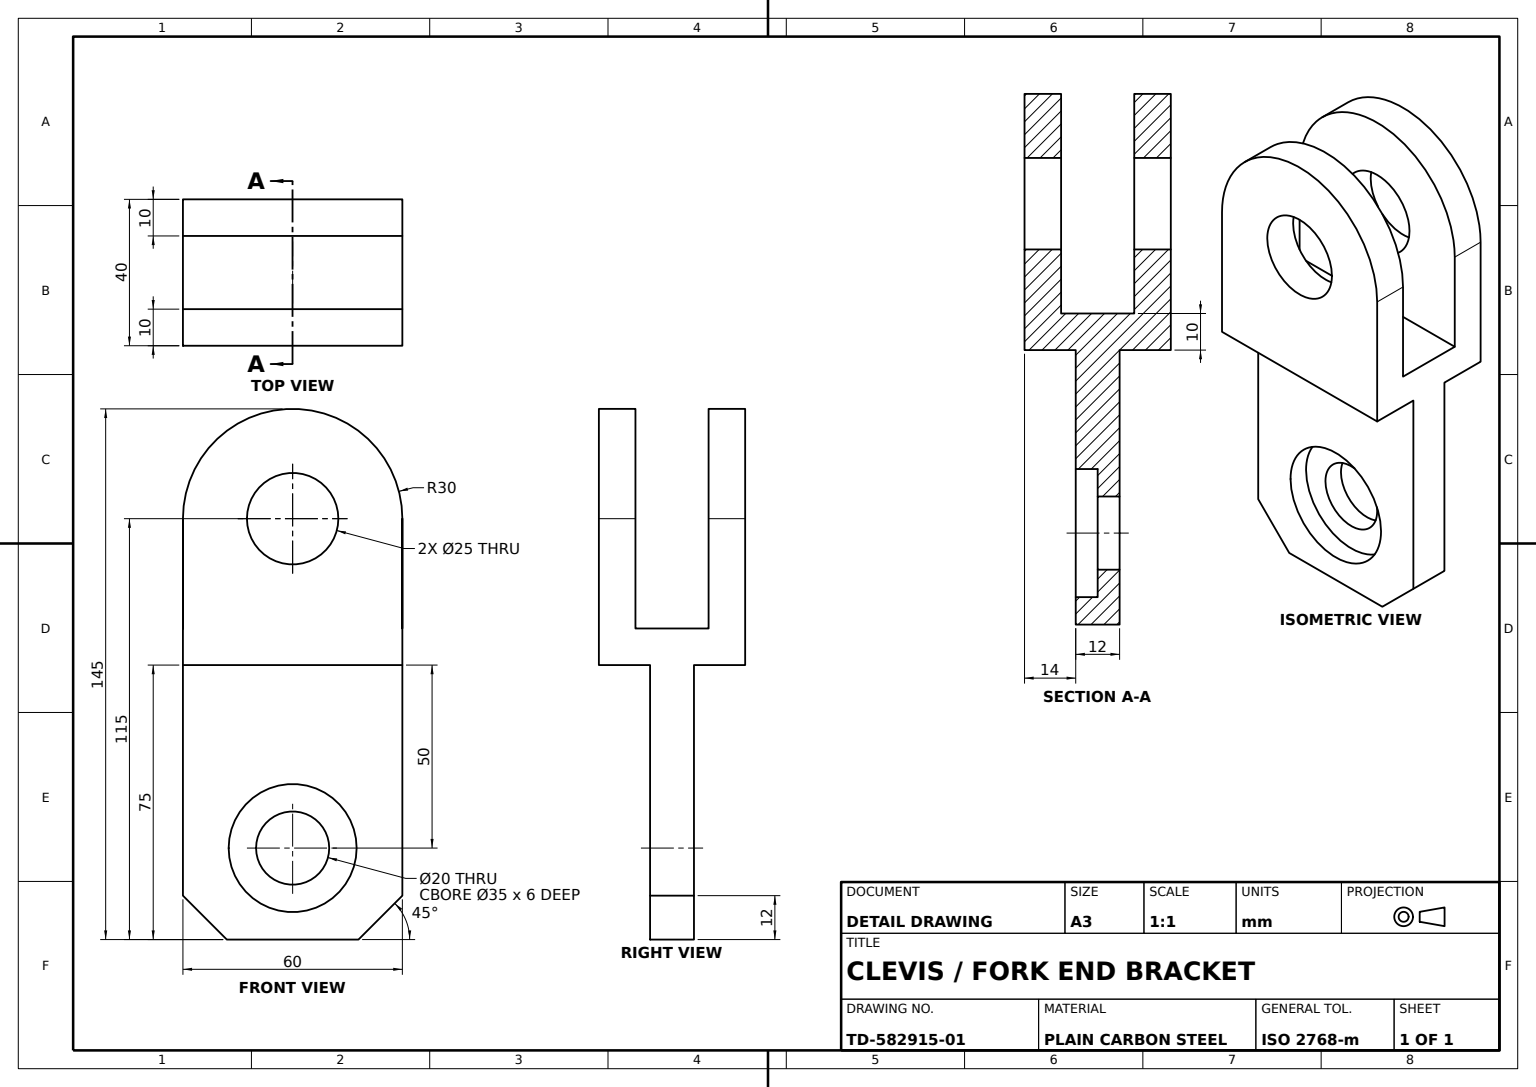
from build123d import *

# Parameters (mm, degrees)
BASE_PLATE_DEPTH       = 12
CLEVIS_BODY_PROFILE_W  = 14
CLEVIS_BODY_PROFILE_H  = 40
CLEVIS_BODY_DEPTH      = 60
CLEVIS_BODY_2_DEPTH    = 60
LUG_1_BOSS_SKETCH_R    = 30
LUG_1_BOSS_DEPTH       = 10
LUG_1_TRIM_SKETCH_W    = 60
LUG_1_TRIM_SKETCH_H    = 4
LUG_1_TRIM_DEPTH       = 40
LUG_2_BOSS_SKETCH_R    = 30
LUG_2_BOSS_DEPTH       = 10
LUG_2_TRIM_SKETCH_W    = 60
LUG_2_TRIM_SKETCH_H    = 4
LUG_2_TRIM_DEPTH       = 40
CLEVIS_WEB_SKETCH_W    = 60
CLEVIS_WEB_SKETCH_H    = 20
CLEVIS_WEB_DEPTH       = 10
PIN_HOLE_SKETCH_R      = 12.5
PIN_HOLE_25_DEPTH      = 40
COUNTERBORE_SKETCH_R   = 17.5
COUNTERBORE_35X6_DEPTH = 6
MOUNTING_HOLE_SKETCH_R = 10
MOUNTING_HOLE_20_DEPTH = 6


with BuildPart() as part:
    # Base Plate Profile → Base Plate (new body)
    with BuildSketch(Plane.XY):
        Polygon((-6, 0), (-6, -63), (6, -75), (42, -75), (54, -63), (54, 0), align=None)
    extrude(amount=BASE_PLATE_DEPTH)



with BuildPart() as body_2:
    # Clevis Body Profile → Clevis Body (new body)
    with BuildSketch(Plane.ZY.offset(6)):
        with Locations((19, 20)):
            Rectangle(CLEVIS_BODY_PROFILE_W, CLEVIS_BODY_PROFILE_H)
    extrude(amount=-CLEVIS_BODY_DEPTH)

    # Lug 2 Boss Sketch → Lug 2 Boss (add)
    with BuildSketch(Plane.XY.offset(26)):
        with Locations((24, 40)):
            Circle(LUG_2_BOSS_SKETCH_R)
    extrude(amount=-LUG_2_BOSS_DEPTH)

    # Lug 2 Trim Sketch → Lug 2 Trim (cut)
    with BuildSketch(Plane(origin=(0, 40, 0), x_dir=(1, 0, 0), z_dir=(0, 1, 0))):
        with Locations((24, -14)):
            Rectangle(LUG_2_TRIM_SKETCH_W, LUG_2_TRIM_SKETCH_H)
    extrude(amount=-LUG_2_TRIM_DEPTH, mode=Mode.SUBTRACT)


with BuildPart() as body_3:
    # Clevis Body Profile → Clevis Body 2 (new body)
    with BuildSketch(Plane.ZY.offset(6)):
        with Locations((-7, 20)):
            Rectangle(CLEVIS_BODY_PROFILE_W, CLEVIS_BODY_PROFILE_H)
    extrude(amount=-CLEVIS_BODY_2_DEPTH)

    # Lug 1 Boss Sketch → Lug 1 Boss (add)
    with BuildSketch(Plane(origin=(0, 0, -14), x_dir=(-1, 0, 0), z_dir=(0, 0, -1))):
        with Locations((-24, 40)):
            Circle(LUG_1_BOSS_SKETCH_R)
    extrude(amount=-LUG_1_BOSS_DEPTH)

    # Lug 1 Trim Sketch → Lug 1 Trim (cut)
    with BuildSketch(Plane(origin=(0, 40, 0), x_dir=(1, 0, 0), z_dir=(0, 1, 0))):
        with Locations((24, 2)):
            Rectangle(LUG_1_TRIM_SKETCH_W, LUG_1_TRIM_SKETCH_H)
    extrude(amount=-LUG_1_TRIM_DEPTH, mode=Mode.SUBTRACT)


with BuildPart() as part_1:
    add(part.part)

    add(body_2.part)  # Clevis Web merges body 2

    add(body_3.part)  # Clevis Web merges body 3
    # Clevis Web Sketch → Clevis Web (add)
    with BuildSketch(Plane(origin=(0, 0, 0), x_dir=(1, 0, 0), z_dir=(0, 1, 0))):
        with Locations((24, -6)):
            Rectangle(CLEVIS_WEB_SKETCH_W, CLEVIS_WEB_SKETCH_H)
    extrude(amount=CLEVIS_WEB_DEPTH)

    # Pin Hole Sketch → Pin Hole Ø25 (cut)
    with BuildSketch(Plane.XY.offset(26)):
        with Locations((24, 40)):
            Circle(PIN_HOLE_SKETCH_R)
    extrude(amount=-PIN_HOLE_25_DEPTH, mode=Mode.SUBTRACT)

    # Counterbore Sketch → Counterbore Ø35x6 (cut)
    with BuildSketch(Plane.XY.offset(12)):
        with Locations((24, -50)):
            Circle(COUNTERBORE_SKETCH_R)
    extrude(amount=-COUNTERBORE_35X6_DEPTH, mode=Mode.SUBTRACT)

    # Mounting Hole Sketch → Mounting Hole Ø20 (cut)
    with BuildSketch(Plane.XY.offset(6)):
        with Locations((24, -50)):
            Circle(MOUNTING_HOLE_SKETCH_R)
    extrude(amount=-MOUNTING_HOLE_20_DEPTH, mode=Mode.SUBTRACT)


solid = part_1.part
